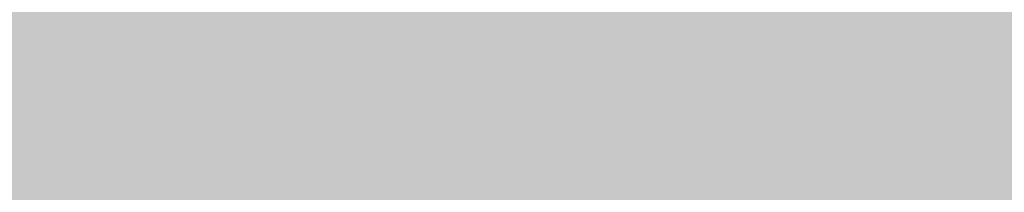
# Model space of a CAD drawing. Units: inches. Extents: x 2091 to 2899, y 967 to 2217.
# Tile 169 of 256: x 2203.14684 to 2203.151632, y 1152.2479 to 1152.248741. Entities that reach past the tile are written whole.
import ezdxf

# ---------------------------------------------------------------- set-up
doc = ezdxf.new("R2010")
doc.units = ezdxf.units.IN
doc.layers.add('A-WALL-PATT', color=141, linetype='Continuous', lineweight=13, true_color=0xadddf7)

msp = doc.modelspace()

# ---------------------------------------------------------------- hatches: boundary and pattern name
at = {"layer": 'A-WALL-PATT'}
h = msp.add_hatch(color=256, dxfattribs=at)
h.dxf.hatch_style = 1
h.paths.add_polyline_path([(2803.1436027, 2050.9190588), (2203.1436027, 2050.9190588), (2203.1436027, 1090.9190588), (2803.1436027, 1090.9190588)])
h.paths.add_polyline_path([(2635.7988501, 1147.5404649), (2674.5240524, 1147.5404649, 0.376086), (2678.5296653, 1152.8802017), (2678.5296653, 1159.5564734, 0.333335), (2674.524319, 1163.561846), (2674.524319, 1163.5618504), (2674.524319, 1192.9343904), (2635.8059707, 1192.9343904), (2597.0876225, 1192.9343904), (2597.0876225, 1163.561846, 0.333335), (2593.0822761, 1159.5564734), (2593.0822761, 1152.8802017, 0.376086), (2597.087889, 1147.5404649)], flags=0)
h.paths.add_polyline_path([(2436.0104329, 1278.2407784, 0.000483), (2435.9526433, 1278.215027, -0.001328), (2435.9356253, 1278.1116934, -0.001711), (2436.1164401, 1278.0407583, 0.002185)], flags=0)
h.paths.add_polyline_path([(2794.1436027, 1143.4190588), (2794.1436027, 1347.4190588), (2543.3701706, 1347.4190588), (2543.3701706, 1351.9190588), (2794.1436027, 1351.9190588), (2794.1436027, 1392.7135549), (2793.9473982, 1392.7135549), (2793.9473982, 1473.5368999), (2794.1436027, 1473.5368999), (2794.1436027, 1531.9190588), (2650.1436027, 1531.9190588), (2650.1436027, 1536.4190588), (2794.1436027, 1536.4190588), (2794.1436027, 1692.4190588), (2609.3756095, 1692.4190588), (2609.3756095, 1644.4190588), (2604.8756095, 1644.4190588), (2604.8756095, 1744.9190588), (2609.3756095, 1744.9190588), (2609.3756095, 1696.9190588), (2794.1436027, 1696.9190588), (2794.1436027, 1780.9190588), (2609.6436027, 1780.9190588), (2493.8756095, 1780.9190588), (2493.8756095, 1785.4190588), (2609.6436027, 1785.4190588), (2794.1436027, 1785.4190588), (2794.1436027, 1847.9388214), (2793.9512217, 1847.9388214), (2793.9512217, 1928.7621663), (2794.1436027, 1928.7621663), (2794.1436027, 1941.4190588), (2614.1436027, 1941.4190588), (2614.1436027, 1821.4190588), (2609.6436027, 1821.4190588), (2609.6436027, 1941.4190588), (2392.1436027, 1941.4190588), (2392.1436027, 1819.9190588), (2387.6436027, 1819.9190588), (2387.6436027, 1941.4190588), (2212.1436027, 1941.4190588), (2212.1436027, 1783.9190588), (2392.1436027, 1783.9190588), (2392.1436027, 1780.9190588), (2212.1436027, 1780.9190588), (2212.1436027, 1629.4190588), (2387.6436027, 1629.4190588), (2387.6436027, 1744.9190588), (2392.1436027, 1744.9190588), (2392.1436027, 1627.9190588), (2317.1436027, 1627.9190588), (2317.1436027, 1551.4190588), (2317.1436027, 1536.4190588), (2459.3835909, 1536.4190588), (2459.3835909, 1602.3964802), (2463.8835909, 1602.3964802), (2463.8835909, 1531.9190588), (2456.6436027, 1531.9190588), (2456.6436027, 1529.9190588), (2452.1436027, 1529.9190588), (2452.1436027, 1531.9190588), (2312.6436027, 1531.9190588), (2312.6436027, 1551.4190588), (2306.1436027, 1551.4190588), (2306.1436027, 1555.9190588), (2308.1436027, 1555.9190588), (2308.1436027, 1551.4190588), (2312.6436027, 1551.4190588), (2312.6436027, 1627.9190588), (2212.1436027, 1627.9190588), (2212.1436027, 1555.9190588), (2270.1436027, 1555.9190588), (2270.1436027, 1551.4190588), (2212.1436027, 1551.4190588), (2212.1436027, 1351.9190588), (2272.1436027, 1351.9190588), (2272.1436027, 1347.4190588), (2212.1436027, 1347.4190588), (2212.1436027, 1275.4190588), (2308.1436027, 1275.4190588), (2308.1436027, 1351.9190588), (2452.1436027, 1351.9190588), (2452.1436027, 1493.9190588), (2456.6436027, 1493.9190588), (2456.6436027, 1347.4190588), (2312.6436027, 1347.4190588), (2312.6436027, 1270.9190588), (2212.1436027, 1270.9190588), (2212.1436027, 1099.9190588), (2281.2375229, 1099.9190588), (2282.8710413, 1110.9138034), (2282.0083413, 1116.9966034), (2278.5577413, 1121.4204034), (2268.2056413, 1128.0562034), (2272.0876413, 1128.0562034), (2273.8129413, 1131.9270034), (2279.4203413, 1134.6919034), (2285.0278413, 1135.2449034), (2287.6158413, 1137.4568034), (2288.0471413, 1138.0098034), (2289.3411413, 1140.7747034), (2291.0665413, 1139.6687034), (2292.3605413, 1135.2449034), (2295.3798413, 1136.9038034), (2296.2425413, 1135.7979034), (2297.1052413, 1133.0330034), (2300.1246413, 1138.0098034), (2303.1439413, 1138.0098034), (2304.4379413, 1135.7979034), (2303.1439413, 1133.5860034), (2306.5946413, 1134.6919034), (2307.8887413, 1133.0330034), (2310.9080413, 1135.2449034), (2313.9274413, 1134.1389034), (2315.6268599, 1132.4271023), (2308.3200413, 1117.5496034), (2290.2038413, 1109.8079034), (2288.9098413, 1103.1721034), (2289.2723086, 1099.9190588), (2434.9182274, 1099.9190588), (2431.5932274, 1124.7880588), (2429.9302274, 1169.5530588), (2430.9271848, 1240.5196942), (2435.6589255, 1238.1861258), (2437.1352274, 1196.5540588), (2438.7982274, 1143.9730588), (2442.6782274, 1111.9980588), (2446.5582274, 1099.9190588), (2794.1436027, 1099.9190588), (2794.1436027, 1138.9190588), (2548.0324471, 1138.9190588), (2548.0324471, 1143.4190588), (2548.0324471, 1148.8190588), (2546.6684571, 1148.0315588), (2528.6856919, 1179.1786218, 0.256256), (2512.0324471, 1148.8190588), (2512.0324471, 1143.4190588), (2512.0324471, 1138.9190588), (2507.5324471, 1138.9190588), (2507.5324471, 1143.4190588), (2507.5324471, 1148.8190588, 0.256256), (2490.8792023, 1179.1786218), (2472.8964371, 1148.0315588), (2471.5324471, 1148.8190588), (2471.5324471, 1143.4190588), (2467.0324471, 1143.4190588), (2467.0324471, 1269.9457858, 0.039061), (2460.9099871, 1273.5800588), (2467.0324471, 1273.5800588), (2467.0324471, 1286.3253638, 0.014511), (2465.2161944, 1286.7619052), (2467.0324471, 1287.0525761), (2467.0324471, 1323.4190588), (2471.5324471, 1323.4190588), (2471.5324471, 1148.8190588), (2489.5324471, 1179.9959734), (2490.8964371, 1179.2084734), (2490.8792023, 1179.1786218, -0.256256), (2507.5324471, 1148.8190588), (2507.5324471, 1143.4190588), (2512.0324471, 1143.4190588), (2512.0324471, 1148.8190588, -0.256256), (2528.6856919, 1179.1786218), (2528.6684571, 1179.2084734), (2530.0324471, 1179.9959734), (2548.0324471, 1148.8190588), (2548.0324471, 1143.4190588)], flags=16)
h.paths.add_polyline_path([(2607.7685461, 1200.9450832), (2607.7685461, 1265.0306251), (2597.0876225, 1281.0520106), (2619.7845852, 1281.0520106), (2627.795278, 1337.1268598), (2635.7988501, 1337.1268598), (2643.8166634, 1337.1268598), (2651.8273562, 1281.0520106), (2674.524319, 1281.0520106), (2663.8433953, 1265.0306251), (2663.8433953, 1200.9450832), (2635.8059707, 1200.9450832)], flags=0)
edge = h.paths.add_edge_path(flags=0)
edge.add_ellipse((13303.8962153, 1272.9987247), major_axis=(-10595.3130399, 0.0000005), ratio=0.842303870086, start_angle=0.62823721906, end_angle=0.64655409989, ccw=False)
edge.add_ellipse((2711.7004495, 1156.8526781), major_axis=(2.2197691, 0), ratio=0.84230387, start_angle=111.5352435, end_angle=180.6282372, ccw=False)
edge.add_ellipse((13303.1562922, 1272.9987246), major_axis=(-10593.0263064, 0), ratio=0.842303869544, start_angle=0.52827147182, end_angle=0.64655409706, ccw=False)
edge.add_line((2710.7645961, 1175.3332951), (2710.1299858, 1175.3332951))
edge.add_ellipse((2710.1299858, 1176.5797752), major_axis=(1.4798461, 0), ratio=0.84230387, start_angle=180, end_angle=270, ccw=False)
edge.add_line((2708.6501397, 1176.5797752), (2708.6501397, 1200.7829144))
edge.add_ellipse((2710.1299858, 1200.7829144), major_axis=(1.4798461, 0), ratio=0.84230387, start_angle=90, end_angle=180, ccw=False)
edge.add_line((2710.1299858, 1202.0293944), (2710.4650752, 1202.0293944))
edge.add_ellipse((13303.1562922, 1272.9987246), major_axis=(-10593.0263064, 0), ratio=0.842303869544, start_angle=-0.09022908859, end_angle=0.38386677879, ccw=False)
edge.add_ellipse((2710.1299858, 1290.9270308), major_axis=(-1.4798461, 0), ratio=0.84230387, start_angle=0, end_angle=90, ccw=False)
edge.add_line((2708.6501397, 1290.9270308), (2708.6501397, 1315.13017))
edge.add_ellipse((2710.1299858, 1315.13017), major_axis=(-1.4798461, 0), ratio=0.84230387, start_angle=-90, end_angle=0, ccw=False)
edge.add_line((2710.1299858, 1316.3766501), (2710.7063141, 1316.3766501))
edge.add_ellipse((3238.4017202, 1296.2895655), major_axis=(528.2339998, 0), ratio=0.84230386954, start_angle=176.349572414, end_angle=177.820049686, ccw=False)
edge.add_ellipse((2775.0630432, 1071.4506962), major_axis=(313.3077613, 0), ratio=0.84230386954, start_angle=102.125965552, end_angle=103.780528989, ccw=False)
edge.add_ellipse((2775.0630432, 1078.3056979), major_axis=(-305.3028915, 0), ratio=0.84230386955, start_angle=-79.790461003, end_angle=-77.555372706, ccw=False)
edge.add_ellipse((2695.1417666, 1541.9753825), major_axis=(-250.9602162, 0), ratio=0.84230386954, start_angle=99.256566007, end_angle=102.554932644)
edge.add_line((2741.4103262, 1334.2142554), (2747.1325454, 1337.3784768))
edge.add_ellipse((2747.5386163, 1336.8574776), major_axis=(-0.739923, 0), ratio=0.84230387, start_angle=270, end_angle=307.9331305, ccw=False)
edge.add_ellipse((2747.5386163, 1336.8574776), major_axis=(-0.739923, 0), ratio=0.84230387, start_angle=232.0668695, end_angle=270, ccw=False)
edge.add_line((2747.9446872, 1337.3784768), (2753.6669064, 1334.2142554))
edge.add_ellipse((2799.935466, 1541.9753825), major_axis=(250.9602162, 0), ratio=0.84230386954, start_angle=257.445067356, end_angle=260.743433993)
edge.add_ellipse((2720.0141894, 1078.3056979), major_axis=(305.3028915, 0), ratio=0.84230386954, start_angle=77.555372707, end_angle=79.790461003, ccw=False)
edge.add_ellipse((2720.0141894, 1071.4506962), major_axis=(-313.3077613, 0), ratio=0.84230386954, start_angle=256.219471011, end_angle=257.874034448, ccw=False)
edge.add_ellipse((2256.6755124, 1296.2895655), major_axis=(-528.2339998, 0), ratio=0.84230386954, start_angle=182.179950314, end_angle=183.650427586, ccw=False)
edge.add_line((2784.3709184, 1316.3766501), (2784.9472468, 1316.3766501))
edge.add_ellipse((2784.9472468, 1315.13017), major_axis=(1.4798461, 0), ratio=0.84230387, start_angle=0, end_angle=90, ccw=False)
edge.add_line((2786.4270928, 1315.13017), (2786.4270928, 1290.9270308))
edge.add_ellipse((2784.9472468, 1290.9270308), major_axis=(1.4798461, 0), ratio=0.84230387, start_angle=270, end_angle=360, ccw=False)
edge.add_ellipse((-7808.0790596, 1272.9987246), major_axis=(10593.0263063, 0), ratio=0.842303869544, start_angle=-0.38386677879, end_angle=0.09022908859, ccw=False)
edge.add_line((2784.6121574, 1202.0293944), (2784.9472468, 1202.0293944))
edge.add_ellipse((2784.9472468, 1200.7829144), major_axis=(1.4798461, 0), ratio=0.84230387, start_angle=0, end_angle=90, ccw=False)
edge.add_line((2786.4270928, 1200.7829144), (2786.4270928, 1176.5797752))
edge.add_ellipse((2784.9472468, 1176.5797752), major_axis=(-1.4798461, 0), ratio=0.84230387, start_angle=90, end_angle=180, ccw=False)
edge.add_line((2784.9472468, 1175.3332951), (2784.3126365, 1175.3332951))
edge.add_ellipse((-7808.0790596, 1272.9987246), major_axis=(10593.0263063, 0), ratio=0.842303869544, start_angle=-0.61864319632, end_angle=-0.52827147182, ccw=False)
edge.add_ellipse((2783.3767831, 1156.8526781), major_axis=(-2.2197691, 0), ratio=0.84230387, start_angle=179.3717628, end_angle=248.4647566, ccw=False)
edge.add_ellipse((-7808.8189826, 1272.9987246), major_axis=(-10595.3130398, 0.0000036), ratio=0.842303865762, start_angle=179.3534459226, end_angle=179.37176280343, ccw=False)
edge.add_ellipse((2780.2973026, 1153.500793), major_axis=(-5.2464256, 0), ratio=0.84230387, start_angle=90, end_angle=179.3534459, ccw=False)
edge.add_line((2780.2973026, 1149.0817084), (2714.77993, 1149.0817084))
edge.add_ellipse((2714.77993, 1153.500793), major_axis=(5.2464256, 0), ratio=0.84230387, start_angle=180.6465541, end_angle=270, ccw=False)
edge = h.paths.add_edge_path(flags=0)
edge.add_line((2718.1873674, 1151.0078329), (2718.1873674, 1170.4723638))
edge.add_ellipse((2721.1470595, 1170.4723638), major_axis=(-2.9596921, 0), ratio=0.84230387, start_angle=-90, end_angle=0, ccw=False)
edge.add_line((2721.1470595, 1172.965324), (2773.9301731, 1172.965324))
edge.add_ellipse((2773.9301731, 1170.4723638), major_axis=(-2.9596921, 0), ratio=0.84230387, start_angle=180, end_angle=270, ccw=False)
edge.add_line((2776.8898652, 1170.4723638), (2776.8898652, 1151.0078329))
edge.add_line((2776.8898652, 1151.0078329), (2718.1873674, 1151.0078329))
edge = h.paths.add_edge_path(flags=0)
edge.add_line((2718.1873674, 1180.2341502), (2718.1873674, 1199.0578342))
edge.add_ellipse((2747.5386163, 1320.3986402), major_axis=(147.0179239, 0), ratio=0.84230386954, start_angle=256.40186531, end_angle=283.59813469)
edge.add_line((2776.8898652, 1199.0578342), (2776.8898652, 1180.2341502))
edge.add_ellipse((2747.5386163, 1301.5749562), major_axis=(147.0179239, 0), ratio=0.84230386954, start_angle=256.40186531, end_angle=283.59813469, ccw=False)
edge = h.paths.add_edge_path(flags=0)
edge.add_ellipse((13303.1562922, 1272.9987246), major_axis=(-10591.5464603, 0), ratio=0.842303869555, start_angle=0.05559431352, end_angle=0.37776419393, ccw=False)
edge.add_line((2711.6168595, 1262.7217103), (2715.6674076, 1249.4953957))
edge.add_ellipse((6413.8919626, 1241.691919), major_axis=(-3698.2361592, 0), ratio=0.842303869547, start_angle=-0.120897369, end_angle=0.3640763489)
edge.add_line((2715.7610383, 1218.1924547), (2711.9343065, 1203.167361))
edge = h.paths.add_edge_path(flags=0)
edge.add_line((2718.1873674, 1251.074566), (2716.0024854, 1267.4504351))
edge.add_ellipse((2742.1511746, 1202.1895399), major_axis=(81.7725845, 0), ratio=0.8423038695, start_angle=94.277420963, end_angle=111.834953797, ccw=False)
edge.add_line((2737.0097482, 1270.9306255), (2758.0674844, 1270.9306255))
edge.add_ellipse((2752.926058, 1202.1895399), major_axis=(81.7725845, 0), ratio=0.8423038695, start_angle=68.165046203, end_angle=85.722579037, ccw=False)
edge.add_line((2779.0747472, 1267.4504351), (2776.8898652, 1251.074566))
edge.add_ellipse((2750.3380588, 1187.8853558), major_axis=(79.5796641, 0), ratio=0.8423038695, start_angle=67.208085122, end_angle=85.129930403)
edge.add_line((2756.0346562, 1254.7436557), (2739.0425764, 1254.7436557))
edge.add_ellipse((2744.7391738, 1187.8853558), major_axis=(79.5796641, 0), ratio=0.8423038695, start_angle=94.870069597, end_angle=112.791914878)
edge = h.paths.add_edge_path(flags=0)
edge.add_line((2783.1429261, 1203.167361), (2779.3161943, 1218.1924547))
edge.add_ellipse((-918.81473, 1241.691919), major_axis=(3698.2361592, 0), ratio=0.842303869546, start_angle=-0.3640763489, end_angle=0.120897369)
edge.add_line((2779.409825, 1249.4953957), (2783.4603731, 1262.7217103))
edge.add_ellipse((-7808.0790596, 1272.9987246), major_axis=(-10591.5464603, 0), ratio=0.84230386954, start_angle=179.6222358061, end_angle=179.94440568651, ccw=False)
edge = h.paths.add_edge_path(flags=0)
edge.add_ellipse((2734.2008921, 1286.6904402), major_axis=(-0.3566086, 6.3400775), ratio=0.603833576, start_angle=89.00201428, end_angle=253.65740805, ccw=False)
edge.add_line((2730.3690013, 1286.5418057), (2730.3690013, 1301.3519803))
edge.add_line((2730.3690013, 1301.3519803), (2735.9133107, 1305.2148028))
edge.add_ellipse((2736.3849168, 1304.7345612), major_axis=(0.739923, 0), ratio=0.84230387, start_angle=90, end_angle=134.4802109, ccw=False)
edge.add_line((2736.3849168, 1305.3578013), (2738.0327829, 1305.3578013))
edge.add_line((2738.0327829, 1305.3578013), (2738.0327829, 1307.7079274))
edge.add_ellipse((2794.201642, 1307.7079274), major_axis=(56.168859, 0), ratio=0.8423038695, start_angle=150.5614304, end_angle=180, ccw=False)
edge.add_ellipse((2700.8755906, 1307.7079274), major_axis=(-56.168859, 0), ratio=0.8423038695, start_angle=180, end_angle=209.4385696, ccw=False)
edge.add_line((2757.0444497, 1307.7079274), (2757.0444497, 1305.3578013))
edge.add_line((2757.0444497, 1305.3578013), (2758.6923157, 1305.3578013))
edge.add_ellipse((2758.6923157, 1304.7345612), major_axis=(-0.739923, 0), ratio=0.84230387, start_angle=225.5197891, end_angle=270, ccw=False)
edge.add_line((2759.1639219, 1305.2148028), (2764.7082312, 1301.3519803))
edge.add_line((2764.7082312, 1301.3519803), (2764.7082312, 1286.5418057))
edge.add_ellipse((2760.8763405, 1286.6904402), major_axis=(0.3566086, 6.3400775), ratio=0.603833576, start_angle=106.34259195, end_angle=270.99798572, ccw=False)
edge.add_line((2757.0444497, 1285.7970896), (2757.0444497, 1307.7079274))
edge.add_ellipse((2700.8755906, 1307.7079274), major_axis=(-56.168859, 0), ratio=0.8423038695, start_angle=180, end_angle=209.4385696)
edge.add_ellipse((2794.201642, 1307.7079274), major_axis=(56.168859, 0), ratio=0.8423038695, start_angle=150.5614304, end_angle=180)
edge.add_line((2738.0327829, 1307.7079274), (2738.0327829, 1285.7970896))
h.paths.add_polyline_path([(2417.8122727, 1104.449704), (2413.4922727, 1102.529704), (2410.6122727, 1103.969704), (2409.1722727, 1106.369704), (2407.2522727, 1107.329704), (2406.2922727, 1109.729704), (2405.3322727, 1114.049704), (2405.3322727, 1117.889704), (2406.2922727, 1120.129704), (2407.2522727, 1119.809704), (2408.8483218, 1118.3276585), (2410.1739451, 1119.4241703), (2410.2112727, 1120.405704), (2411.0407305, 1121.4190541), (2410.6992727, 1119.858704), (2410.1739451, 1119.4241703), (2410.0884515, 1117.1761095), (2411.1328361, 1116.2063237), (2413.9722727, 1119.329704), (2416.8522727, 1120.769704), (2416.8697209, 1120.7987842), (2417.0350713, 1119.4051162), (2417.8962134, 1118.1433844), (2418.2922727, 1118.369704), (2419.5444467, 1120.0392692), (2419.3609153, 1118.387487), (2419.0321078, 1119.3561507), (2418.3989394, 1118.5119262), (2419.2522727, 1114.529704), (2418.7940909, 1107.1987949)], flags=0)
h.paths.add_polyline_path([(2508.8701706, 1347.4190588), (2508.3701706, 1347.4190588), (2508.3701706, 1351.9190588), (2508.8701706, 1351.9190588)], flags=0)
h.paths.add_polyline_path([(2473.3701706, 1347.4190588), (2472.3701706, 1347.4190588), (2467.8701706, 1347.4190588), (2467.8701706, 1455.4190588), (2472.3701706, 1455.4190588), (2472.3701706, 1352.4190588), (2473.3701706, 1352.4190588)], flags=0)
h.paths.add_polyline_path([(2352.106244, 1217.4461971), (2349.226244, 1218.8861971), (2347.786244, 1221.2861971), (2345.866244, 1222.2461971), (2344.906244, 1224.6461971), (2343.946244, 1228.9661971), (2343.946244, 1232.8061971), (2344.906244, 1235.0461971), (2345.866244, 1234.7261971), (2347.4622931, 1233.2441515), (2348.7879164, 1234.3406634), (2348.825244, 1235.3221971), (2349.6547018, 1236.3355471), (2349.313244, 1234.7751971), (2348.7879164, 1234.3406634), (2348.7024228, 1232.0926025), (2349.7468074, 1231.1228168), (2352.586244, 1234.2461971), (2355.466244, 1235.6861971), (2355.4836921, 1235.7152773), (2355.6490426, 1234.3216093), (2356.5101846, 1233.0598774), (2356.906244, 1233.2861971), (2358.1584179, 1234.9557623), (2357.9748866, 1233.3039801), (2357.6460791, 1234.2726438), (2357.0129107, 1233.4284193), (2357.866244, 1229.4461971), (2357.4080622, 1222.115288), (2356.426244, 1219.3661971)], flags=0)
h.paths.add_polyline_path([(2348.2967999, 1112.2244204), (2347.0137999, 1112.3104204), (2345.5297999, 1114.1274204), (2345.7317999, 1115.8584204), (2346.8117999, 1116.9824204), (2346.8117999, 1114.6464204), (2345.8667999, 1114.2144204), (2346.8797999, 1114.3004204)], flags=0)
h.paths.add_polyline_path([(2347.0137999, 1110.9264204), (2346.2717999, 1110.4934204), (2346.6097999, 1111.1864204)], flags=0)
h.paths.add_polyline_path([(2345.8667999, 1118.1944204), (2345.5297999, 1117.3294204), (2343.7077999, 1118.0214204), (2344.3827999, 1118.6264204)], flags=0)
h.paths.add_polyline_path([(2346.6767999, 1109.2824204), (2346.0697999, 1108.0714204), (2345.8667999, 1110.0614204)], flags=0)
h.paths.add_polyline_path([(2345.0567999, 1119.7514204), (2343.6397999, 1119.7514204), (2343.9777999, 1121.1354204)], flags=0)
h.paths.add_polyline_path([(2345.2597999, 1116.5504204), (2345.1247999, 1115.8584204), (2344.9217999, 1115.6854204), (2344.7197999, 1116.3774204)], flags=0)
h.paths.add_polyline_path([(2345.6647999, 1112.3104204), (2345.4617999, 1111.5324204), (2344.0447999, 1111.9644204), (2344.6517999, 1112.5704204)], flags=0)
h.paths.add_polyline_path([(2345.1917999, 1113.3494204), (2344.4497999, 1113.8684204), (2344.7197999, 1114.3874204)], flags=0)
h.paths.add_polyline_path([(2344.6517999, 1116.8094204), (2344.1797999, 1115.6854204), (2344.6517999, 1115.3394204), (2343.9097999, 1114.9064204), (2343.0327999, 1115.9444204), (2343.6397999, 1116.4634204)], flags=0)
h.paths.add_polyline_path([(2345.8667999, 1106.6864204), (2344.9897999, 1105.5624204), (2344.5167999, 1106.6004204)], flags=0)
h.paths.add_polyline_path([(2344.8547999, 1110.0614204), (2344.5167999, 1109.2824204), (2344.1127999, 1109.7154204)], flags=0)
h.paths.add_polyline_path([(2344.0447999, 1113.5224204), (2343.4377999, 1113.0894204), (2342.7627999, 1113.9544204)], flags=0)
h.paths.add_polyline_path([(2344.3147999, 1111.0124204), (2342.9647999, 1110.3204204), (2342.9647999, 1111.0994204)], flags=0)
h.paths.add_polyline_path([(2345.1247999, 1104.6974204), (2344.5847999, 1103.7454204), (2344.4497999, 1104.2644204)], flags=0)
h.paths.add_polyline_path([(2342.8297999, 1121.2224204), (2341.7497999, 1120.5304204), (2340.5357999, 1121.0494204), (2340.1307999, 1121.8284204), (2340.6707999, 1122.9524204), (2341.1427999, 1121.8284204), (2341.6147999, 1122.0014204)], flags=0)
h.paths.add_polyline_path([(2342.9647999, 1119.7514204), (2343.0327999, 1118.4534204), (2342.0877999, 1118.0214204), (2342.0197999, 1119.4914204)], flags=0)
h.paths.add_polyline_path([(2342.6947999, 1116.8964204), (2341.9527999, 1116.6364204), (2342.0197999, 1117.3294204)], flags=0)
h.paths.add_polyline_path([(2343.0327999, 1112.2244204), (2342.0197999, 1111.7914204), (2341.5477999, 1112.2244204), (2342.3577999, 1113.3494204)], flags=0)
h.paths.add_polyline_path([(2343.7747999, 1104.4374204), (2342.6277999, 1102.8804204), (2342.6947999, 1104.6104204), (2343.4377999, 1105.1294204)], flags=0)
h.paths.add_polyline_path([(2342.0197999, 1115.0794204), (2340.8057999, 1115.5124204), (2340.9407999, 1116.3774204)], flags=0)
h.paths.add_polyline_path([(2341.4807999, 1120.0974204), (2341.4807999, 1119.4054204), (2341.0757999, 1119.5784204), (2341.1427999, 1120.0974204)], flags=0)
h.paths.add_polyline_path([(2341.8177999, 1114.4734204), (2340.9407999, 1113.0894204), (2340.8057999, 1114.5604204)], flags=0)
h.paths.add_polyline_path([(2341.1427999, 1118.5404204), (2340.9407999, 1116.9824204), (2339.0507999, 1117.6754204), (2339.0507999, 1118.6264204)], flags=0)
h.paths.add_polyline_path([(2342.6947999, 1101.6684204), (2341.9527999, 1101.8414204), (2342.5597999, 1102.3614204)], flags=0)
h.paths.add_polyline_path([(2340.3327999, 1119.6654204), (2338.4437999, 1119.5784204), (2337.9037999, 1120.3574204), (2339.6577999, 1120.6164204)], flags=0)
h.paths.add_polyline_path([(2340.3327999, 1115.3394204), (2340.0627999, 1113.6954204), (2339.3877999, 1115.3394204)], flags=0)
h.paths.add_polyline_path([(2341.8177999, 1103.8314204), (2341.5477999, 1102.8804204), (2341.1427999, 1103.6584204)], flags=0)
h.paths.add_polyline_path([(2339.0507999, 1122.8664204), (2337.2957999, 1121.8284204), (2337.0937999, 1123.1254204), (2337.7687999, 1123.8184204)], flags=0)
h.paths.add_polyline_path([(2339.1177999, 1121.7414204), (2338.8477999, 1121.2224204), (2338.1737999, 1121.0494204), (2338.3757999, 1121.5684204)], flags=0)
h.paths.add_polyline_path([(2339.1857999, 1119.3194204), (2338.6457999, 1118.7134204), (2338.2407999, 1118.1074204), (2338.2407999, 1118.8864204)], flags=0)
h.paths.add_polyline_path([(2341.1427999, 1101.9284204), (2340.6027999, 1101.2364204), (2340.0627999, 1101.8414204), (2340.6027999, 1102.3614204)], flags=0)
h.paths.add_polyline_path([(2337.6337999, 1117.7614204), (2336.6207999, 1118.2804204), (2337.2957999, 1118.9724204)], flags=0)
h.paths.add_polyline_path([(2336.8237999, 1119.5784204), (2334.7987999, 1118.9724204), (2335.2037999, 1120.3574204), (2336.5537999, 1120.8764204)], flags=0)
h.paths.add_polyline_path([(2339.1177999, 1100.4574204), (2337.3637999, 1100.5434204), (2336.7557999, 1101.2364204)], flags=0)
h.paths.add_polyline_path([(2336.3507999, 1122.4334204), (2336.0137999, 1121.9144204), (2334.9337999, 1122.4334204), (2334.5287999, 1123.4714204), (2335.7437999, 1122.7794204)], flags=0)
h.paths.add_polyline_path([(2334.7317999, 1120.8764204), (2334.2587999, 1120.3574204), (2334.0567999, 1120.7894204), (2334.5967999, 1121.3084204)], flags=0)
h.paths.add_polyline_path([(2334.4617999, 1122.1744204), (2332.5717999, 1121.3084204), (2331.3567999, 1122.1744204), (2332.0997999, 1122.8664204)], flags=0)
h.paths.add_polyline_path([(2334.2587999, 1118.5404204), (2333.3817999, 1118.4534204), (2333.6517999, 1119.3194204)], flags=0)
h.paths.add_polyline_path([(2335.5417999, 1102.2744204), (2334.1917999, 1102.6204204), (2335.2717999, 1103.3124204)], flags=0)
h.paths.add_polyline_path([(2332.7067999, 1119.6654204), (2331.6947999, 1120.4434204), (2332.5047999, 1120.7894204)], flags=0)
h.paths.add_polyline_path([(2334.7317999, 1101.1494204), (2333.5167999, 1101.5824204), (2333.9887999, 1101.7554204)], flags=0)
h.paths.add_polyline_path([(2332.6397999, 1116.6364204), (2331.0867999, 1116.2904204), (2331.9647999, 1118.1944204)], flags=0)
h.paths.add_polyline_path([(2330.7497999, 1121.5684204), (2330.2767999, 1120.2704204), (2328.5227999, 1119.3194204), (2328.9947999, 1121.0494204)], flags=0)
h.paths.add_polyline_path([(2330.7497999, 1118.6264204), (2330.0077999, 1117.5024204), (2329.8727999, 1118.0214204)], flags=0)
h.paths.add_polyline_path([(2332.0997999, 1102.3614204), (2330.5467999, 1102.0144204), (2331.6947999, 1102.9664204)], flags=0)
h.paths.add_polyline_path([(2329.5347999, 1113.6084204), (2329.0627999, 1112.3104204), (2328.5897999, 1113.3494204)], flags=0)
h.paths.add_polyline_path([(2328.3877999, 1117.8484204), (2327.5097999, 1116.5504204), (2327.1727999, 1117.7614204)], flags=0)
h.paths.add_polyline_path([(2329.7377999, 1106.5134204), (2329.5347999, 1105.3024204), (2328.2527999, 1106.0814204)], flags=0)
h.paths.add_polyline_path([(2328.6577999, 1114.3874204), (2328.0497999, 1114.1274204), (2328.3197999, 1114.9064204)], flags=0)
h.paths.add_polyline_path([(2328.3197999, 1112.2244204), (2327.1057999, 1112.1374204), (2326.7007999, 1112.6564204)], flags=0)
h.paths.add_polyline_path([(2326.9027999, 1115.2524204), (2326.7007999, 1114.1274204), (2325.2157999, 1113.6084204), (2326.0927999, 1115.3394204)], flags=0)
h.paths.add_polyline_path([(2326.6327999, 1108.3304204), (2326.0927999, 1107.3794204), (2325.8907999, 1108.5034204), (2326.4977999, 1109.1094204)], flags=0)
h.paths.add_polyline_path([(2615.1436027, 1531.9190588), (2609.6436027, 1531.9190588), (2609.6436027, 1620.4190588), (2614.1436027, 1620.4190588), (2614.1436027, 1536.4190588), (2615.1436027, 1536.4190588)], flags=0)
h.paths.add_polyline_path([(2545.1436027, 1563.4190588), (2464.1436027, 1563.4190588), (2464.1436027, 1632.4190588), (2509.1436027, 1632.4190588), (2509.1436027, 1627.9190588), (2509.1436027, 1603.9190588), (2468.6436027, 1603.9190588), (2468.6436027, 1567.9190588), (2540.6436027, 1567.9190588), (2540.6436027, 1591.9190588), (2545.1436027, 1591.9190588)], flags=0)
h.paths.add_polyline_path([(2388.9690483, 1549.985735), (2357.4341811, 1549.985735), (2357.4341811, 1623.3607783), (2399.3627772, 1623.3607783), (2435.6894654, 1623.3607783), (2435.5925469, 1602.5592734), (2435.5925469, 1602.3964802), (2388.9690483, 1602.3964802)], flags=0)
h.paths.add_polyline_path([(2388.8806282, 1555.8091511), (2374.9044295, 1555.8091511), (2374.9044295, 1600.5715641), (2374.9044295, 1615.4576454), (2406.3508766, 1615.4576454), (2406.3508766, 1618.9394309), (2412.1742927, 1615.4576454), (2406.3508766, 1611.9758599), (2406.3508766, 1615.4576454), (2388.8806282, 1615.4576454)], flags=0)
h.paths.add_polyline_path([(2568.8756095, 1644.4190588), (2453.3756095, 1644.4190588), (2453.3756095, 1785.4190588), (2457.8756095, 1785.4190588), (2457.8756095, 1648.9190588), (2568.8756095, 1648.9190588)], flags=0)
h.paths.add_polyline_path([(2212.1436027, 1945.9190588), (2212.1436027, 2041.9190588), (2794.1436027, 2041.9190588), (2794.1436027, 1945.9190588)], flags=16)
h.paths.add_polyline_path([(2271.0827276, 1964.3172377), (2776.852968, 1964.3172377), (2776.852968, 2037.1696226), (2271.0827276, 2037.1696226)], flags=8)
h.paths.add_polyline_path([(2380.6492852, 1536.8241435), (2461.0408087, 1536.8241435), (2461.0408087, 1554.6525871), (2380.6492852, 1554.6525871)], flags=8)
h.paths.add_polyline_path([(2240.7557092, 1609.7254508), (2309.1858294, 1609.7254508), (2309.1858294, 1617.6982037), (2240.7557092, 1617.6982037)], flags=8)
h.paths.add_polyline_path([(2212.6772554, 1313.5041021), (2282.5915203, 1313.5041021), (2282.5915203, 1322.7452389), (2212.6772554, 1322.7452389)], flags=8)
h.paths.add_polyline_path([(2457.111976, 1114.778574), (2558.4815807, 1114.778574), (2558.4815807, 1142.2196823), (2457.111976, 1142.2196823)], flags=8)
h.paths.add_polyline_path([(2473.4423372, 1273.0100672), (2604.6412257, 1273.0100672), (2604.6412257, 1318.3469349), (2473.4423372, 1318.3469349)], flags=8)
h.paths.add_polyline_path([(2638.8763024, 1626.9774316), (2684.2503675, 1627.9767377), (2684.0384825, 1637.5974944), (2638.6644174, 1636.5981884)], flags=8)
h.paths.add_polyline_path([(2537.5905538, 1453.7934466), (2628.3895472, 1453.7934466), (2628.3895472, 1475.3448114), (2537.5905538, 1475.3448114)], flags=8)
h.paths.add_polyline_path([(2504.1376376, 1714.6323972), (2554.6471875, 1714.6323972), (2554.6471875, 1730.2377115), (2504.1376376, 1730.2377115)], flags=8)
h.paths.add_polyline_path([(2487.5011806, 1575.6518716), (2535.0971214, 1575.6518716), (2535.0971214, 1598.3776456), (2487.5011806, 1598.3776456)], flags=8)
h.paths.add_polyline_path([(2709.0994004, 1735.7102784), (2740.0166009, 1735.7102784), (2740.0166009, 1749.9376406), (2709.0994004, 1749.9376406)], flags=8)
h.paths.add_polyline_path([(2442.4384239, 1792.1716575), (2564.7288353, 1792.1716575), (2564.7288353, 1842.0001626), (2442.4384239, 1842.0001626)], flags=8)
h.paths.add_polyline_path([(2655.8158012, 1809.6440763), (2789.5201425, 1806.6937963), (2790.0849768, 1832.2916379), (2656.3806355, 1835.2419179)], flags=8)
h.paths.add_polyline_path([(2234.8426972, 1797.7201432), (2368.5928512, 1794.7688523), (2369.1607182, 1820.504132), (2235.4105642, 1823.4554229)], flags=8)
h.paths.add_polyline_path([(2245.1384659, 1644.0063348), (2398.4277329, 1640.6238997), (2398.9948417, 1666.3248199), (2245.7055747, 1669.7072549)], flags=8)
h.paths.add_polyline_path([(2306.1428474, 1431.1685186), (2413.7683138, 1428.7936873), (2414.3331481, 1454.3915289), (2306.7076817, 1456.7663602)], flags=8)
h.paths.add_polyline_path([(2306.834582, 1458.2331447), (2393.3804836, 1456.3234487), (2393.9328082, 1481.3543583), (2307.3869066, 1483.2640542)], flags=8)

doc.saveas('drawing.dxf')
